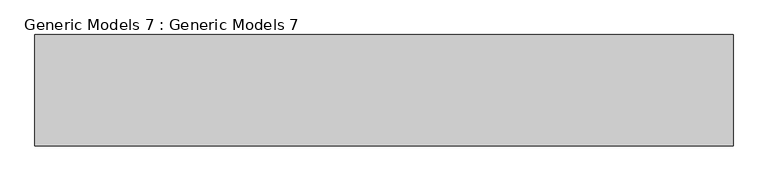
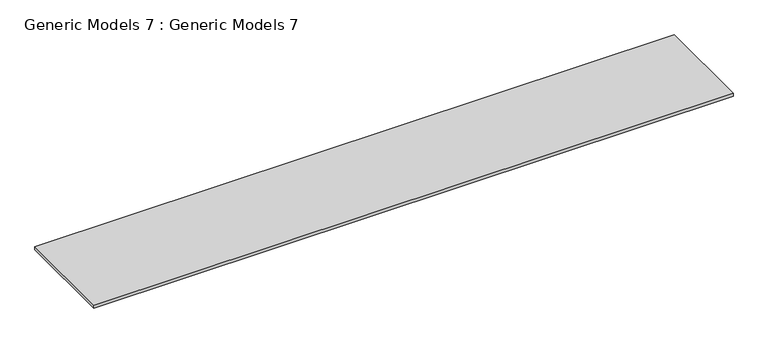
"""IFC4 building model written with IfcOpenShell, lengths in millimetres: proxy geometry, Generic Models 7 : Generic Models 7."""

from ifc_helpers import new_model, si_unit, frame, origin, place, context, project, spatial, polyline, outline, extrude, source, transform, mapped, element, save


def generic_models_7_generic_models_7_4119f6ec(model_context):
    return source(origin(), model_context, "Body", "SweptSolid", [
        extrude(outline(polyline([(-16131.8645113, -18613.3447932), (-16131.8645113, -13553.5007495), (15567.3354887, -13553.5007495), (15567.3354887, -18613.3447932), (-16131.8645113, -18613.3447932)])), frame((0.0, 0.0, -152.4), z_axis=(0.0, 0.0, 1.0), x_axis=(1.0, 0.0, 0.0)), (0.0, 0.0, 1.0), 152.4),
    ])


if __name__ == "__main__":
    model = new_model("IFC4")
    model_context = context("Model", 3, world=origin())
    ifc_project = project(units=[si_unit("LENGTHUNIT", "METRE", prefix="MILLI")], contexts=[model_context])
    site = spatial("IfcSite", under=ifc_project)
    building = spatial("IfcBuilding", under=site)
    placement = place(None, origin())
    generic_models_7_generic_models_7_shape = generic_models_7_generic_models_7_4119f6ec(model_context)
    element("IfcBuildingElementProxy", 1, Name="Generic Models 7 : Generic Models 7", ObjectType="Generic Models 7 : Generic Models 7", at=placement, inside=building, context=model_context, shape_type="MappedRepresentation", body=[
        mapped(generic_models_7_generic_models_7_shape, transform((0.0, 0.0, 0.0), x_axis=(1.0, 0.0, 0.0), y_axis=(0.0, 1.0, 0.0), z_axis=(0.0, 0.0, 1.0))),
    ])
    save(model, "model.ifc")
